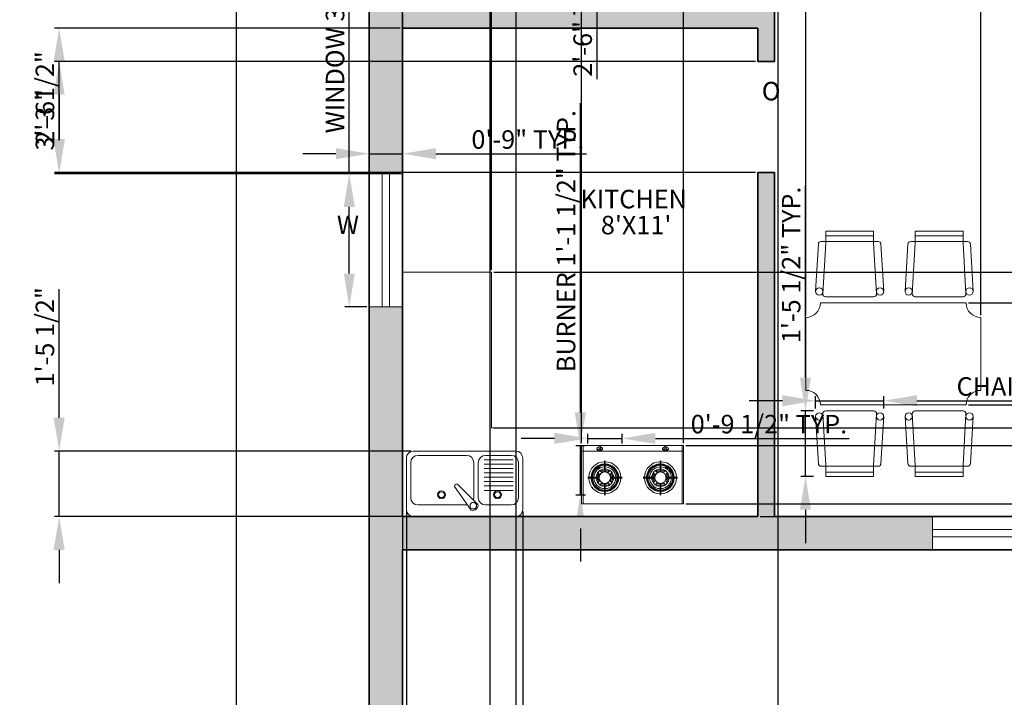
# Model space of a CAD drawing. Units: inches. Extents: x 2265 to 2807, y 1544 to 2401.
# Tile 2 of 9: x 2265 to 2531, y 1890 to 2073. Entities that reach past the tile are written whole.
import ezdxf

# ---------------------------------------------------------------- set-up
doc = ezdxf.new("R2010")
doc.units = ezdxf.units.IN
for name, color, linetype, lineweight in [('A-ANNO-DIMS', 2, 'Continuous', 18), ('A-ANNO-TEXT', 7, 'Continuous', 18), ('A-AREA-IDEN', 7, 'Continuous', 18), ('A-EQPM', 8, 'Continuous', 15), ('A-FLOR-CASE', 8, 'Continuous', 20), ('A-FLOR-FIXT', 8, 'Continuous', 18), ('A-GLAZ', 4, 'Continuous', 18), ('A-WALL', 7, 'Continuous', 35), ('A-WALL-PATT', 18, 'Continuous', 13), ('C-PROP', 7, 'Continuous', 25), ('Furniture', 161, 'Continuous', 15)]:
    doc.layers.add(name, color=color, linetype=linetype, lineweight=lineweight)
doc.styles.add('ARIAL', font='times.ttf', dxfattribs={"height": 5})
doc.styles.get("Standard").update_dxf_attribs({"font": 'arial.ttf', "height": 5})
doc.dimstyles.new('ISO-25', dxfattribs={"dimtxt": 5, "dimasz": 9, "dimexe": 1.25, "dimexo": 0.625, "dimtad": 1, "dimlunit": 3, "dimtxsty": 'Standard', "dimcen": 2.5, "dimadec": 0, "dimazin": 0, "dimtfac": 1, "dimtmove": 0, "dimatfit": 3, "dimfxl": 1, "dimarcsym": 0})

# ---------------------------------------------------------------- blocks, each defined once
blk = doc.blocks.new('GLAZING-48IN')
for p, q in [((48, 9), (0, 9)), ((0, 5.5), (48, 5.5)), ((0, 5.5), (48, 5.5)), ((0, 3.5), (48, 3.5)), ((0, 0), (48, 0))]:
    blk.add_line(p, q)
blk = doc.blocks.new('GLAZING-36IN')
for p, q in [((0, 36), (0, 0)), ((3.5, 36), (3.5, 0)), ((5.5, 36), (5.5, 0)), ((5.5, 36), (5.5, 0)), ((9, 0), (9, 36))]:
    blk.add_line(p, q)
blk = doc.blocks.new('DINING-CHAIR')
for p, q in [((0, 16.18), (0.74, 3.5)), ((1.93, 16.88), (2.73, 3.09)), ((2.72, 17.72), (15.66, 17.72)), ((16.45, 16.88), (15.65, 3.09)), ((18.38, 16.18), (17.65, 3.5)), ((1.52, 2.76), (16.86, 2.76)), ((2.72, 0), (2.73, 3.09)), ((15.66, 0), (15.65, 3.09)), ((2.72, 1.18), (15.66, 1.18)), ((2.72, 0), (15.66, 0))]:
    blk.add_line(p, q)
for centre in [(0.98, 16.24), (17.39, 16.24)]:
    blk.add_circle(centre, 0.984)
for centre, start, end in [((2.72, 16.93), 90, 183.3132), ((15.66, 16.93), 356.6868, 90), ((1.52, 3.54), 183.3132, 270), ((1.52, 3.54), 183.3132, 270), ((16.86, 3.54), 270, 356.6868)]:
    blk.add_arc(centre, 0.787, start, end)
blk = doc.blocks.new('HOB-BURNER-CONTROL')
for p, q in [((2.48, 12.56), (2.48, 12.42)), ((3.09, 13.22), (3.09, 12.56)), ((3.09, 12.56), (3.09, 12.34)), ((3.36, 13.3), (3.17, 13.3)), ((3.17, 12.48), (3.36, 12.48)), ((3.44, 12.56), (3.44, 13.22)), ((3.44, 12.56), (3.44, 12.34)), ((4.03, 12.56), (4.03, 12.42)), ((4.54, 6.45), (4.54, 9.28)), ((4.73, 6.45), (4.73, 9.28)), ((2.54, 5.77), (2.75, 5.57)), ((2.71, 6.05), (3.13, 5.62)), ((3.27, 6.61), (3.69, 6.18)), ((3.54, 6.78), (3.75, 6.57)), ((5.73, 6.78), (5.52, 6.57)), ((6, 6.61), (5.58, 6.18)), ((6.56, 6.05), (6.13, 5.62)), ((6.73, 5.77), (6.52, 5.57)), ((2.87, 4.78), (0, 4.78)), ((2.87, 4.58), (0, 4.58)), ((2.75, 3.79), (2.54, 3.59)), ((3.13, 3.74), (2.71, 3.31)), ((3.69, 3.18), (3.27, 2.76)), ((3.75, 2.79), (3.54, 2.59)), ((4.54, 2.91), (4.54, 0)), ((4.73, 2.91), (4.73, 0)), ((5.52, 2.79), (5.73, 2.59)), ((5.58, 3.18), (6, 2.76)), ((6.13, 3.74), (6.56, 3.31)), ((6.4, 4.78), (9.3, 4.78)), ((6.4, 4.58), (9.3, 4.58)), ((6.52, 3.79), (6.73, 3.59))]:
    blk.add_line(p, q)
for centre, radius in [((2.72, 7.23), 0.141), ((3.08, 7.46), 0.141), ((4.63, 4.68), 1.54)]:
    blk.add_circle(centre, radius)
for centre, radius, start, end in [((2.55, 12.57), 0.0787, 165.3271, 228.6514), ((3.25, 13.37), 1.14, 228.6514, 256.6925), ((3.01, 12.34), 0.0787, 256.6925, 0), ((3.17, 13.22), 0.0787, 90, 180), ((3.17, 12.56), 0.0787, 180, 270), ((3.36, 13.22), 0.0787, 0, 90), ((3.36, 12.56), 0.0787, 270, 0), ((3.52, 12.34), 0.0787, 180, 284.376), ((3.25, 13.37), 1.14, 284.376, 309.6111), ((3.93, 12.58), 0.104, 300.0749, 32.1858), ((4.63, 4.68), 4.33, 91.3023, 178.6977), ((4.63, 4.68), 3.74, 91.5918, 178.4082), ((4.63, 4.68), 3.54, 91.5918, 178.4082), ((4.63, 4.68), 3.35, 91.6854, 178.3146), ((4.63, 4.68), 4.33, 1.3023, 88.6977), ((4.63, 4.68), 3.54, 1.5918, 88.4082), ((4.63, 4.68), 3.35, 1.6854, 88.3146), ((4.63, 4.68), 3.74, 1.5918, 88.4082), ((4.63, 4.68), 2.95, 91.9102, 178.0898), ((4.63, 4.68), 2.36, 92.388, 177.612), ((4.63, 4.68), 2.09, 154.8539, 177.2964), ((4.63, 4.68), 1.77, 147.8396, 176.8153), ((4.63, 4.68), 1.77, 93.1847, 122.1604), ((4.63, 4.68), 2.09, 92.7036, 115.1461), ((4.63, 6.48), 0.104, 198.751, 341.249), ((4.63, 4.68), 2.95, 1.9102, 88.0898), ((4.63, 4.68), 2.36, 2.388, 87.612), ((4.63, 4.68), 2.09, 64.8539, 87.2964), ((4.63, 4.68), 1.77, 57.8396, 86.8153), ((4.63, 4.68), 1.77, 3.1847, 32.1604), ((4.63, 4.68), 2.09, 2.7036, 25.1461), ((4.63, 4.68), 4.33, 181.3023, 268.6977), ((4.63, 4.68), 3.74, 181.5918, 268.4082), ((4.63, 4.68), 3.54, 181.5918, 268.4082), ((4.63, 4.68), 3.35, 181.6854, 268.3146), ((4.63, 4.68), 2.95, 181.9102, 268.0898), ((4.63, 4.68), 2.36, 182.388, 267.612), ((4.63, 4.68), 2.09, 182.7036, 205.1461), ((2.85, 4.68), 0.0991, 276.7354, 83.2646), ((4.63, 4.68), 1.77, 183.1847, 212.1604), ((4.63, 4.68), 1.77, 237.8396, 266.8153), ((4.63, 4.68), 2.09, 244.8539, 267.2964), ((4.63, 2.88), 0.105, 20.5507, 159.4493), ((4.63, 4.68), 4.33, 271.3023, 358.6977), ((4.63, 4.68), 3.54, 271.5918, 358.4082), ((4.63, 4.68), 3.35, 271.6854, 358.3146), ((4.63, 4.68), 2.36, 272.388, 357.612), ((4.63, 4.68), 2.95, 271.9102, 358.0898), ((4.63, 4.68), 1.77, 273.1847, 302.1604), ((4.63, 4.68), 2.09, 272.7036, 295.1461), ((4.63, 4.68), 3.74, 271.5918, 358.4082), ((4.63, 4.68), 1.77, 327.8396, 356.8153), ((6.44, 4.68), 0.106, 111.7885, 248.2115), ((4.63, 4.68), 2.09, 334.8539, 357.2964)]:
    blk.add_arc(centre, radius, start, end)
at = {"extrusion": (0, 0, -1)}
for start_param, end_param in [(0.167831, 1.359229), (3.311147, 6.113631), (1.807364, 2.885846)]:
    blk.add_ellipse((3.25, 12.51), major_axis=(-0.788, 0), ratio=0.647058, start_param=start_param, end_param=end_param, dxfattribs=at)
blk = doc.blocks.new('*D17')
at = {"layer": 'A-ANNO-DIMS', "color": 0, "lineweight": -2, "transparency": 16777216}
for p, q in [((2353.7, 2031.88), (2353.7, 2105.4)), ((2358.48, 2031.88), (2352.45, 2031.88)), ((2353.7, 2004.88), (2353.7, 2022.88)), ((2358.48, 1995.88), (2352.45, 1995.88))]:
    blk.add_line(p, q, dxfattribs=at)
at = {"layer": 'A-ANNO-DIMS', "color": 0, "lineweight": 100, "transparency": 16777216}
for points in [[(2352.2, 2022.88), (2355.2, 2022.88), (2353.7, 2031.88)], [(2352.2, 2004.88), (2355.2, 2004.88), (2353.7, 1995.88)]]:
    blk.add_solid(points, dxfattribs=at)
at = {"layer": 'Defpoints', "color": 0, "lineweight": 100, "transparency": 16777216}
for p in [(2353.7, 2031.88), (2359.1, 2031.88), (2359.1, 1995.88)]:
    blk.add_point(p, dxfattribs=at)
at = {"layer": 'A-ANNO-DIMS', "color": 0, "transparency": 16777216, "insert": (2350.49, 2073.14), "char_height": 5, "attachment_point": 5, "rotation": 90}
blk.add_mtext('WINDOW 3\'-0" TYP.', dxfattribs=at)
blk = doc.blocks.new('*D18')
at = {"layer": 'A-ANNO-DIMS', "color": 0, "lineweight": -2, "transparency": 16777216}
for p, q in [((2359.1, 2032.51), (2359.1, 2038.53)), ((2368.1, 2032.51), (2368.1, 2038.53)), ((2350.1, 2037.28), (2341.1, 2037.28)), ((2359.1, 2037.28), (2368.1, 2037.28)), ((2377.1, 2037.28), (2417.83, 2037.28))]:
    blk.add_line(p, q, dxfattribs=at)
at = {"layer": 'A-ANNO-DIMS', "color": 0, "lineweight": 100, "transparency": 16777216}
for points in [[(2350.1, 2038.78), (2350.1, 2035.78), (2359.1, 2037.28)], [(2377.1, 2038.78), (2377.1, 2035.78), (2368.1, 2037.28)]]:
    blk.add_solid(points, dxfattribs=at)
at = {"layer": 'Defpoints', "color": 0, "lineweight": 100, "transparency": 16777216}
for p in [(2368.1, 2037.28), (2359.1, 2031.88), (2368.1, 2031.88)]:
    blk.add_point(p, dxfattribs=at)
at = {"layer": 'A-ANNO-DIMS', "color": 0, "transparency": 16777216, "insert": (2401.96, 2040.46), "char_height": 5, "attachment_point": 5}
blk.add_mtext('0\'-9" TYP.', dxfattribs=at)
blk = doc.blocks.new('*D24')
at = {"layer": 'A-ANNO-DIMS', "color": 0, "lineweight": -2, "transparency": 16777216}
for p, q in [((2424.48, 2128.23), (2419.35, 2128.23)), ((2420.6, 2119.23), (2420.6, 2107.23)), ((2424.48, 2098.23), (2419.35, 2098.23)), ((2420.6, 2098.23), (2420.6, 2057.42))]:
    blk.add_line(p, q, dxfattribs=at)
at = {"layer": 'A-ANNO-DIMS', "color": 0, "lineweight": 100, "transparency": 16777216}
for points in [[(2419.1, 2119.23), (2422.1, 2119.23), (2420.6, 2128.23)], [(2419.1, 2107.23), (2422.1, 2107.23), (2420.6, 2098.23)]]:
    blk.add_solid(points, dxfattribs=at)
at = {"layer": 'Defpoints', "color": 0, "lineweight": 100, "transparency": 16777216}
for p in [(2425.1, 2128.23), (2420.6, 2098.23), (2425.1, 2098.23)]:
    blk.add_point(p, dxfattribs=at)
at = {"layer": 'A-ANNO-DIMS', "color": 0, "transparency": 16777216, "insert": (2417.42, 2073.33), "char_height": 5, "attachment_point": 5, "rotation": 90}
blk.add_mtext('2\'-6" TYP.', dxfattribs=at)
blk = doc.blocks.new('*D27')
at = {"layer": 'A-ANNO-DIMS', "color": 0, "lineweight": -2, "transparency": 16777216}
for p, q in [((2470.74, 1970.54), (2461.74, 1970.54)), ((2479.74, 1968.41), (2479.74, 1971.79)), ((2479.74, 1970.54), (2498.12, 1970.54)), ((2498.12, 1968.41), (2498.12, 1971.79)), ((2507.12, 1970.54), (2583.11, 1970.54))]:
    blk.add_line(p, q, dxfattribs=at)
at = {"layer": 'A-ANNO-DIMS', "color": 0, "lineweight": 100, "transparency": 16777216}
for points in [[(2470.74, 1972.04), (2470.74, 1969.04), (2479.74, 1970.54)], [(2507.12, 1972.04), (2507.12, 1969.04), (2498.12, 1970.54)]]:
    blk.add_solid(points, dxfattribs=at)
at = {"layer": 'Defpoints', "color": 0, "lineweight": 100, "transparency": 16777216}
for p in [(2498.12, 1970.54), (2479.74, 1967.79), (2498.12, 1967.79)]:
    blk.add_point(p, dxfattribs=at)
at = {"layer": 'A-ANNO-DIMS', "color": 0, "transparency": 16777216, "insert": (2549.62, 1973.75), "char_height": 5, "attachment_point": 5}
blk.add_mtext('CHAIR 1\'-6 1/2" TYP.', dxfattribs=at)
blk = doc.blocks.new('*D28')
at = {"layer": 'A-ANNO-DIMS', "color": 0, "lineweight": -2, "transparency": 16777216}
for p, q in [((2476.98, 1976.79), (2476.98, 2028.69)), ((2479.11, 1967.79), (2475.73, 1967.79)), ((2476.98, 1950.07), (2476.98, 1967.79)), ((2479.11, 1950.07), (2475.73, 1950.07)), ((2476.98, 1941.07), (2476.98, 1932.07))]:
    blk.add_line(p, q, dxfattribs=at)
at = {"layer": 'A-ANNO-DIMS', "color": 0, "lineweight": 100, "transparency": 16777216}
for points in [[(2475.48, 1976.79), (2478.48, 1976.79), (2476.98, 1967.79)], [(2475.48, 1941.07), (2478.48, 1941.07), (2476.98, 1950.07)]]:
    blk.add_solid(points, dxfattribs=at)
at = {"layer": 'Defpoints', "color": 0, "lineweight": 100, "transparency": 16777216}
for p in [(2476.98, 1967.79), (2479.74, 1967.79), (2479.74, 1950.07)]:
    blk.add_point(p, dxfattribs=at)
at = {"layer": 'A-ANNO-DIMS', "color": 0, "transparency": 16777216, "insert": (2473.77, 2007.24), "char_height": 5, "attachment_point": 5, "rotation": 90}
blk.add_mtext('1\'-5 1/2" TYP.', dxfattribs=at)
blk = doc.blocks.new('*D33')
at = {"layer": 'A-ANNO-DIMS', "color": 0, "lineweight": -2, "transparency": 16777216}
for p, q in [((2416.14, 1967.36), (2416.14, 2050.96)), ((2417.51, 1958.36), (2414.89, 1958.36)), ((2416.14, 1945.06), (2416.14, 1958.36)), ((2417.51, 1945.06), (2414.89, 1945.06)), ((2416.14, 1936.06), (2416.14, 1927.06))]:
    blk.add_line(p, q, dxfattribs=at)
at = {"layer": 'A-ANNO-DIMS', "color": 0, "lineweight": 100, "transparency": 16777216}
for points in [[(2414.64, 1967.36), (2417.64, 1967.36), (2416.14, 1958.36)], [(2414.64, 1936.06), (2417.64, 1936.06), (2416.14, 1945.06)]]:
    blk.add_solid(points, dxfattribs=at)
at = {"layer": 'Defpoints', "color": 0, "lineweight": 100, "transparency": 16777216}
for p in [(2416.14, 1958.36), (2418.13, 1958.36), (2418.13, 1945.06)]:
    blk.add_point(p, dxfattribs=at)
at = {"layer": 'A-ANNO-DIMS', "color": 0, "transparency": 16777216, "insert": (2412.93, 2013.66), "char_height": 5, "attachment_point": 5, "rotation": 90}
blk.add_mtext('BURNER 1\'-1 1/2" TYP.', dxfattribs=at)
blk = doc.blocks.new('*D34')
at = {"layer": 'A-ANNO-DIMS', "color": 0, "lineweight": -2, "transparency": 16777216}
for p, q in [((2418.13, 1958.99), (2418.13, 1961.61)), ((2427.43, 1958.99), (2427.43, 1961.61)), ((2409.13, 1960.36), (2400.13, 1960.36)), ((2418.13, 1960.36), (2427.43, 1960.36)), ((2436.43, 1960.36), (2488.81, 1960.36))]:
    blk.add_line(p, q, dxfattribs=at)
at = {"layer": 'A-ANNO-DIMS', "color": 0, "lineweight": 100, "transparency": 16777216}
for points in [[(2409.13, 1961.86), (2409.13, 1958.86), (2418.13, 1960.36)], [(2436.43, 1961.86), (2436.43, 1958.86), (2427.43, 1960.36)]]:
    blk.add_solid(points, dxfattribs=at)
at = {"layer": 'Defpoints', "color": 0, "lineweight": 100, "transparency": 16777216}
for p in [(2427.43, 1960.36), (2418.13, 1958.36), (2427.43, 1958.36)]:
    blk.add_point(p, dxfattribs=at)
at = {"layer": 'A-ANNO-DIMS', "color": 0, "transparency": 16777216, "insert": (2467.12, 1963.57), "char_height": 5, "attachment_point": 5}
blk.add_mtext('0\'-9 1/2" TYP.', dxfattribs=at)
blk = doc.blocks.new('*D37')
at = {"layer": 'A-ANNO-DIMS', "color": 0, "lineweight": -2, "transparency": 16777216}
for p, q in [((2463.48, 2062.23), (2274.04, 2062.23)), ((2275.29, 2053.23), (2275.29, 2041.23)), ((2463.48, 2032.23), (2274.04, 2032.23))]:
    blk.add_line(p, q, dxfattribs=at)
at = {"layer": 'A-ANNO-DIMS', "color": 0, "lineweight": 100, "transparency": 16777216}
for points in [[(2273.79, 2053.23), (2276.79, 2053.23), (2275.29, 2062.23)], [(2273.79, 2041.23), (2276.79, 2041.23), (2275.29, 2032.23)]]:
    blk.add_solid(points, dxfattribs=at)
at = {"layer": 'Defpoints', "color": 0, "lineweight": 100, "transparency": 16777216}
for p in [(2464.1, 2062.23), (2275.29, 2032.23), (2464.1, 2032.23)]:
    blk.add_point(p, dxfattribs=at)
at = {"layer": 'A-ANNO-DIMS', "color": 0, "transparency": 16777216, "insert": (2272.11, 2047.23), "char_height": 5, "attachment_point": 5, "rotation": 90}
blk.add_mtext('2\'-6"', dxfattribs=at)
blk = doc.blocks.new('*D40')
at = {"layer": 'A-ANNO-DIMS', "color": 0, "lineweight": -2, "transparency": 16777216}
for p, q in [((2368.1, 2005.86), (2368.1, 2297.59)), ((2392.1, 2005.86), (2392.1, 2297.59)), ((2377.1, 2296.34), (2383.1, 2296.34))]:
    blk.add_line(p, q, dxfattribs=at)
at = {"layer": 'A-ANNO-DIMS', "color": 0, "lineweight": 100, "transparency": 16777216}
for points in [[(2377.1, 2297.84), (2377.1, 2294.84), (2368.1, 2296.34)], [(2383.1, 2297.84), (2383.1, 2294.84), (2392.1, 2296.34)]]:
    blk.add_solid(points, dxfattribs=at)
at = {"layer": 'Defpoints', "color": 0, "lineweight": 100, "transparency": 16777216}
for p in [(2392.1, 2296.34), (2368.1, 2005.23), (2392.1, 2005.23)]:
    blk.add_point(p, dxfattribs=at)
at = {"layer": 'A-ANNO-DIMS', "color": 0, "transparency": 16777216, "insert": (2380.1, 2299.52), "char_height": 5, "attachment_point": 5}
blk.add_mtext('2\'-0"', dxfattribs=at)
blk = doc.blocks.new('*D41')
at = {"layer": 'A-ANNO-DIMS', "color": 0, "lineweight": -2, "transparency": 16777216}
for p, q in [((2392.73, 2005.23), (2804.46, 2005.23)), ((2803.21, 1996.23), (2803.21, 1972.23)), ((2392.73, 1963.23), (2804.46, 1963.23))]:
    blk.add_line(p, q, dxfattribs=at)
at = {"layer": 'A-ANNO-DIMS', "color": 0, "lineweight": 100, "transparency": 16777216}
for points in [[(2801.71, 1996.23), (2804.71, 1996.23), (2803.21, 2005.23)], [(2801.71, 1972.23), (2804.71, 1972.23), (2803.21, 1963.23)]]:
    blk.add_solid(points, dxfattribs=at)
at = {"layer": 'Defpoints', "color": 0, "lineweight": 100, "transparency": 16777216}
for p in [(2392.1, 2005.23), (2392.1, 1963.23), (2803.21, 1963.23)]:
    blk.add_point(p, dxfattribs=at)
at = {"layer": 'A-ANNO-DIMS', "color": 0, "transparency": 16777216, "insert": (2800.03, 1984.23), "char_height": 5, "attachment_point": 5, "rotation": 90}
blk.add_mtext('3\'-6"', dxfattribs=at)
blk = doc.blocks.new('*D42')
at = {"layer": 'A-ANNO-DIMS', "color": 0, "lineweight": -2, "transparency": 16777216}
for p, q in [((2464.73, 1963.23), (2804.46, 1963.23)), ((2803.21, 1954.23), (2803.21, 1948.23)), ((2464.73, 1939.23), (2804.46, 1939.23))]:
    blk.add_line(p, q, dxfattribs=at)
at = {"layer": 'A-ANNO-DIMS', "color": 0, "lineweight": 100, "transparency": 16777216}
for points in [[(2801.71, 1954.23), (2804.71, 1954.23), (2803.21, 1963.23)], [(2801.71, 1948.23), (2804.71, 1948.23), (2803.21, 1939.23)]]:
    blk.add_solid(points, dxfattribs=at)
at = {"layer": 'Defpoints', "color": 0, "lineweight": 100, "transparency": 16777216}
for p in [(2464.1, 1963.23), (2464.1, 1939.23), (2803.21, 1939.23)]:
    blk.add_point(p, dxfattribs=at)
at = {"layer": 'A-ANNO-DIMS', "color": 0, "transparency": 16777216, "insert": (2800.03, 1951.23), "char_height": 5, "attachment_point": 5, "rotation": 90}
blk.add_mtext('2\'-0"', dxfattribs=at)
blk = doc.blocks.new('*D43')
at = {"layer": 'A-ANNO-DIMS', "color": 0, "lineweight": -2, "transparency": 16777216}
for p, q in [((2416.49, 1959.08), (2416.49, 2297.59)), ((2444.05, 1959.08), (2444.05, 2297.59)), ((2425.49, 2296.34), (2435.05, 2296.34))]:
    blk.add_line(p, q, dxfattribs=at)
at = {"layer": 'A-ANNO-DIMS', "color": 0, "lineweight": 100, "transparency": 16777216}
for points in [[(2425.49, 2297.84), (2425.49, 2294.84), (2416.49, 2296.34)], [(2435.05, 2297.84), (2435.05, 2294.84), (2444.05, 2296.34)]]:
    blk.add_solid(points, dxfattribs=at)
at = {"layer": 'Defpoints', "color": 0, "lineweight": 100, "transparency": 16777216}
for p in [(2444.05, 2296.34), (2416.49, 1958.45), (2444.05, 1958.45)]:
    blk.add_point(p, dxfattribs=at)
at = {"layer": 'A-ANNO-DIMS', "color": 0, "transparency": 16777216, "insert": (2430.27, 2299.56), "char_height": 5, "attachment_point": 5}
blk.add_mtext('2\'-3 1/2"', dxfattribs=at)
blk = doc.blocks.new('*D44')
at = {"layer": 'A-ANNO-DIMS', "color": 0, "lineweight": -2, "transparency": 16777216}
for p, q in [((2369.12, 1940.58), (2369.12, 1546.93)), ((2400.62, 1940.58), (2400.62, 1546.93)), ((2378.12, 1548.18), (2391.62, 1548.18))]:
    blk.add_line(p, q, dxfattribs=at)
at = {"layer": 'A-ANNO-DIMS', "color": 0, "lineweight": 100, "transparency": 16777216}
for points in [[(2378.12, 1549.68), (2378.12, 1546.68), (2369.12, 1548.18)], [(2391.62, 1549.68), (2391.62, 1546.68), (2400.62, 1548.18)]]:
    blk.add_solid(points, dxfattribs=at)
at = {"layer": 'Defpoints', "color": 0, "lineweight": 100, "transparency": 16777216}
for p in [(2369.12, 1941.2), (2400.62, 1941.2), (2400.62, 1548.18)]:
    blk.add_point(p, dxfattribs=at)
at = {"layer": 'A-ANNO-DIMS', "color": 0, "transparency": 16777216, "insert": (2384.87, 1551.4), "char_height": 5, "attachment_point": 5}
blk.add_mtext('2\'-7 1/2"', dxfattribs=at)
blk = doc.blocks.new('*D45')
at = {"layer": 'A-ANNO-DIMS', "color": 0, "lineweight": -2, "transparency": 16777216}
for p, q in [((2391.72, 2088.38), (2391.72, 1546.93)), ((2368.1, 2075.11), (2368.1, 1546.93)), ((2377.1, 1548.18), (2382.72, 1548.18)), ((2391.72, 1548.18), (2430.33, 1548.18))]:
    blk.add_line(p, q, dxfattribs=at)
at = {"layer": 'A-ANNO-DIMS', "color": 0, "lineweight": 100, "transparency": 16777216}
for points in [[(2377.1, 1549.68), (2377.1, 1546.68), (2368.1, 1548.18)], [(2382.72, 1549.68), (2382.72, 1546.68), (2391.72, 1548.18)]]:
    blk.add_solid(points, dxfattribs=at)
at = {"layer": 'Defpoints', "color": 0, "lineweight": 100, "transparency": 16777216}
for p in [(2391.72, 2089), (2368.1, 2075.73), (2391.72, 1548.18)]:
    blk.add_point(p, dxfattribs=at)
at = {"layer": 'A-ANNO-DIMS', "color": 0, "transparency": 16777216, "insert": (2415.53, 1551.4), "char_height": 5, "attachment_point": 5}
blk.add_mtext('1\'-11 1/2"', dxfattribs=at)
blk = doc.blocks.new('*D46')
at = {"layer": 'A-ANNO-DIMS', "color": 0, "lineweight": -2, "transparency": 16777216}
for p, q in [((2803.21, 2104.95), (2803.21, 2128.02)), ((2381.23, 2095.95), (2804.46, 2095.95)), ((2803.21, 2082.06), (2803.21, 2095.95)), ((2381.23, 2082.06), (2804.46, 2082.06)), ((2803.21, 2073.06), (2803.21, 2064.06))]:
    blk.add_line(p, q, dxfattribs=at)
at = {"layer": 'A-ANNO-DIMS', "color": 0, "lineweight": 100, "transparency": 16777216}
for points in [[(2801.71, 2104.95), (2804.71, 2104.95), (2803.21, 2095.95)], [(2801.71, 2073.06), (2804.71, 2073.06), (2803.21, 2082.06)]]:
    blk.add_solid(points, dxfattribs=at)
at = {"layer": 'Defpoints', "color": 0, "lineweight": 100, "transparency": 16777216}
for p in [(2380.61, 2095.95), (2803.21, 2095.95), (2380.61, 2082.06)]:
    blk.add_point(p, dxfattribs=at)
at = {"layer": 'A-ANNO-DIMS', "color": 0, "transparency": 16777216, "insert": (2800.07, 2120.99), "char_height": 5, "attachment_point": 5, "rotation": 90}
blk.add_mtext('1\'-2"', dxfattribs=at)
blk = doc.blocks.new('*D48')
at = {"layer": 'A-ANNO-DIMS', "color": 0, "lineweight": -2, "transparency": 16777216}
for p, q in [((2367.48, 2071.23), (2274.04, 2071.23)), ((2275.29, 2040.88), (2275.29, 2062.23)), ((2367.48, 2031.88), (2274.04, 2031.88))]:
    blk.add_line(p, q, dxfattribs=at)
at = {"layer": 'A-ANNO-DIMS', "color": 0, "lineweight": 100, "transparency": 16777216}
for points in [[(2273.79, 2062.23), (2276.79, 2062.23), (2275.29, 2071.23)], [(2273.79, 2040.88), (2276.79, 2040.88), (2275.29, 2031.88)]]:
    blk.add_solid(points, dxfattribs=at)
at = {"layer": 'Defpoints', "color": 0, "lineweight": 100, "transparency": 16777216}
for p in [(2275.29, 2071.23), (2368.1, 2071.23), (2368.1, 2031.88)]:
    blk.add_point(p, dxfattribs=at)
at = {"layer": 'A-ANNO-DIMS', "color": 0, "transparency": 16777216, "insert": (2272.08, 2051.56), "char_height": 5, "attachment_point": 5, "rotation": 90}
blk.add_mtext('3\'-3 1/2"', dxfattribs=at)
blk = doc.blocks.new('*D50')
at = {"layer": 'A-ANNO-DIMS', "color": 0, "lineweight": -2, "transparency": 16777216}
for p, q in [((2398.67, 2169.19), (2398.67, 1546.93)), ((2469.53, 2169.19), (2469.53, 1546.93)), ((2407.67, 1548.18), (2460.53, 1548.18))]:
    blk.add_line(p, q, dxfattribs=at)
at = {"layer": 'A-ANNO-DIMS', "color": 0, "lineweight": 100, "transparency": 16777216}
for points in [[(2407.67, 1549.68), (2407.67, 1546.68), (2398.67, 1548.18)], [(2460.53, 1549.68), (2460.53, 1546.68), (2469.53, 1548.18)]]:
    blk.add_solid(points, dxfattribs=at)
at = {"layer": 'Defpoints', "color": 0, "lineweight": 100, "transparency": 16777216}
for p in [(2398.67, 2169.81), (2469.53, 2169.81), (2469.53, 1548.18)]:
    blk.add_point(p, dxfattribs=at)
at = {"layer": 'A-ANNO-DIMS', "color": 0, "transparency": 16777216, "insert": (2434.1, 1551.36), "char_height": 5, "attachment_point": 5}
blk.add_mtext('5\'-11"', dxfattribs=at)
blk = doc.blocks.new('*D61')
at = {"layer": 'A-ANNO-DIMS', "color": 0, "lineweight": -2, "transparency": 16777216}
for p, q in [((2803.21, 1967.45), (2803.21, 1976.45)), ((2444.67, 1958.45), (2804.46, 1958.45)), ((2803.21, 1958.45), (2803.21, 1942.7)), ((2444.67, 1942.7), (2804.46, 1942.7)), ((2803.21, 1933.7), (2803.21, 1898.98))]:
    blk.add_line(p, q, dxfattribs=at)
at = {"layer": 'A-ANNO-DIMS', "color": 0, "lineweight": 100, "transparency": 16777216}
for points in [[(2801.71, 1967.45), (2804.71, 1967.45), (2803.21, 1958.45)], [(2801.71, 1933.7), (2804.71, 1933.7), (2803.21, 1942.7)]]:
    blk.add_solid(points, dxfattribs=at)
at = {"layer": 'Defpoints', "color": 0, "lineweight": 100, "transparency": 16777216}
for p in [(2444.05, 1958.45), (2444.05, 1942.7), (2803.21, 1942.7)]:
    blk.add_point(p, dxfattribs=at)
at = {"layer": 'A-ANNO-DIMS', "color": 0, "transparency": 16777216, "insert": (2800, 1911.84), "char_height": 5, "attachment_point": 5, "rotation": 90}
blk.add_mtext('1\'-3 1/2"', dxfattribs=at)
blk = doc.blocks.new('*D62')
at = {"layer": 'A-ANNO-DIMS', "color": 0, "lineweight": -2, "transparency": 16777216}
for p, q in [((2275.29, 1965.95), (2275.29, 2000.67)), ((2370.46, 1956.95), (2274.04, 1956.95)), ((2275.29, 1939.23), (2275.29, 1956.95)), ((2370.46, 1939.23), (2274.04, 1939.23)), ((2275.29, 1930.23), (2275.29, 1921.23))]:
    blk.add_line(p, q, dxfattribs=at)
at = {"layer": 'A-ANNO-DIMS', "color": 0, "lineweight": 100, "transparency": 16777216}
for points in [[(2273.79, 1965.95), (2276.79, 1965.95), (2275.29, 1956.95)], [(2273.79, 1930.23), (2276.79, 1930.23), (2275.29, 1939.23)]]:
    blk.add_solid(points, dxfattribs=at)
at = {"layer": 'Defpoints', "color": 0, "lineweight": 100, "transparency": 16777216}
for p in [(2275.29, 1956.95), (2371.09, 1956.95), (2371.09, 1939.23)]:
    blk.add_point(p, dxfattribs=at)
at = {"layer": 'A-ANNO-DIMS', "color": 0, "transparency": 16777216, "insert": (2272.08, 1987.81), "char_height": 5, "attachment_point": 5, "rotation": 90}
blk.add_mtext('1\'-5 1/2"', dxfattribs=at)
blk = doc.blocks.new('*D63')
at = {"layer": 'A-ANNO-DIMS', "color": 0, "lineweight": -2, "transparency": 16777216}
for p, q in [((2477.1, 1993.66), (2477.1, 2297.59)), ((2524.34, 1993.66), (2524.34, 2297.59)), ((2486.1, 2296.34), (2515.34, 2296.34))]:
    blk.add_line(p, q, dxfattribs=at)
at = {"layer": 'A-ANNO-DIMS', "color": 0, "lineweight": 100, "transparency": 16777216}
for points in [[(2486.1, 2297.84), (2486.1, 2294.84), (2477.1, 2296.34)], [(2515.34, 2297.84), (2515.34, 2294.84), (2524.34, 2296.34)]]:
    blk.add_solid(points, dxfattribs=at)
at = {"layer": 'Defpoints', "color": 0, "lineweight": 100, "transparency": 16777216}
for p in [(2524.34, 2296.34), (2477.1, 1993.03), (2524.34, 1993.03)]:
    blk.add_point(p, dxfattribs=at)
at = {"layer": 'A-ANNO-DIMS', "color": 0, "transparency": 16777216, "insert": (2500.72, 2299.52), "char_height": 5, "attachment_point": 5}
blk.add_mtext('3\'-11"', dxfattribs=at)
blk = doc.blocks.new('*D64')
at = {"layer": 'A-ANNO-DIMS', "color": 0, "lineweight": -2, "transparency": 16777216}
for p, q in [((2521.03, 1996.97), (2804.46, 1996.97)), ((2803.21, 1978.41), (2803.21, 1987.97)), ((2521.03, 1969.41), (2804.46, 1969.41))]:
    blk.add_line(p, q, dxfattribs=at)
at = {"layer": 'A-ANNO-DIMS', "color": 0, "lineweight": 100, "transparency": 16777216}
for points in [[(2801.71, 1987.97), (2804.71, 1987.97), (2803.21, 1996.97)], [(2801.71, 1978.41), (2804.71, 1978.41), (2803.21, 1969.41)]]:
    blk.add_solid(points, dxfattribs=at)
at = {"layer": 'Defpoints', "color": 0, "lineweight": 100, "transparency": 16777216}
for p in [(2520.4, 1996.97), (2803.21, 1996.97), (2520.4, 1969.41)]:
    blk.add_point(p, dxfattribs=at)
at = {"layer": 'A-ANNO-DIMS', "color": 0, "transparency": 16777216, "insert": (2800, 1983.19), "char_height": 5, "attachment_point": 5, "rotation": 90}
blk.add_mtext('2\'-3 1/2"', dxfattribs=at)

msp = doc.modelspace()

# ---------------------------------------------------------------- hatches: boundary and pattern name
at = {"layer": 'A-WALL-PATT'}
h = msp.add_hatch(color=256, dxfattribs=at)
h.dxf.hatch_style = 1
h.paths.add_polyline_path([(2416.101, 2255.733), (2359.101, 2255.733), (2359.101, 2205.483), (2368.101, 2205.483), (2368.101, 2246.733), (2416.101, 2246.733)])
h.paths.add_polyline_path([(2528.601, 2255.733), (2452.101, 2255.733), (2452.101, 2246.733), (2487.251, 2246.733), (2500.101, 2246.733), (2500.101, 2168.733), (2504.601, 2168.733), (2504.601, 2170.233), (2525.601, 2170.233), (2525.601, 2174.733), (2504.601, 2174.733), (2504.601, 2246.733), (2528.601, 2246.733)])
h.paths.add_polyline_path([(2603.601, 2255.733), (2552.601, 2255.733), (2552.601, 2246.733), (2576.601, 2246.733), (2576.601, 2174.733), (2555.601, 2174.733), (2555.601, 2170.233), (2576.601, 2170.233), (2576.601, 2123.733), (2581.101, 2123.733), (2581.101, 2246.733), (2603.601, 2246.733)])
h.paths.add_polyline_path([(2671.101, 2255.733), (2639.601, 2255.733), (2639.601, 2246.733), (2662.101, 2246.733), (2662.101, 2083.435), (2671.101, 2083.435)])
h.paths.add_polyline_path([(2671.101, 2035.435), (2662.101, 2035.435), (2662.101, 1939.233), (2644.101, 1939.233), (2644.101, 1930.233), (2662.101, 1930.233), (2662.101, 1814.733), (2644.101, 1814.733), (2644.101, 1805.733), (2671.101, 1805.733)])
h.paths.add_polyline_path([(2368.101, 1930.233), (2511.351, 1930.233), (2511.351, 1939.233), (2468.601, 1939.233), (2468.601, 2032.233), (2464.101, 2032.233), (2464.101, 1939.233), (2368.101, 1939.233), (2368.101, 1995.884), (2359.101, 1995.884), (2359.101, 1805.733), (2602.101, 1805.733), (2602.101, 1814.733), (2368.101, 1814.733)])
h.paths.add_polyline_path([(2368.101, 2071.233), (2464.101, 2071.233), (2464.101, 2062.233), (2468.601, 2062.233), (2468.601, 2123.733), (2504.601, 2123.733), (2504.601, 2132.733), (2500.101, 2132.733), (2500.101, 2128.233), (2455.101, 2128.233), (2455.101, 2123.733), (2464.101, 2123.733), (2464.101, 2075.733), (2368.101, 2075.733), (2368.101, 2087.733), (2359.101, 2087.733), (2359.101, 2031.884), (2368.101, 2031.884)])
h.paths.add_polyline_path([(2368.101, 2169.483), (2359.101, 2169.483), (2359.101, 2111.733), (2368.101, 2111.733), (2368.101, 2123.733), (2425.101, 2123.733), (2425.101, 2128.233), (2368.101, 2128.233)])

# ---------------------------------------------------------------- linework, layer by layer
at = {"layer": 'A-EQPM'}
for p, q in [((2416.49, 1958.452), (2416.49, 1942.704)), ((2444.049, 1958.452), (2416.49, 1958.452)), ((2444.049, 1956.877), (2416.49, 1956.877)), ((2416.884, 1958.452), (2416.884, 1942.704)), ((2443.656, 1942.704), (2443.656, 1958.452)), ((2444.049, 1942.704), (2444.049, 1958.452)), ((2416.49, 1942.704), (2444.049, 1942.704))]:
    msp.add_line(p, q, dxfattribs=at)
at = {"layer": 'A-FLOR-CASE'}
for p, q in [((2392.101, 2005.233), (2368.101, 2005.233)), ((2392.101, 1963.233), (2392.101, 2005.233)), ((2464.101, 1963.233), (2392.101, 1963.233))]:
    msp.add_line(p, q, dxfattribs=at)
at = {"layer": 'A-FLOR-FIXT'}
for p, q in [((2398.647, 1956.95), (2371.088, 1956.95)), ((2369.119, 1954.981), (2369.119, 1941.202)), ((2370.3, 1953.8), (2370.3, 1944.351)), ((2385.407, 1955.769), (2372.269, 1955.769)), ((2387.375, 1944.351), (2387.375, 1953.8)), ((2388.556, 1944.351), (2388.556, 1953.8)), ((2390.14, 1954.594), (2398.028, 1954.594)), ((2390.14, 1953.413), (2398.028, 1953.413)), ((2397.466, 1955.769), (2390.525, 1955.769)), ((2399.434, 1944.351), (2399.434, 1953.8)), ((2400.615, 1941.202), (2400.615, 1954.981)), ((2390.14, 1952.232), (2398.028, 1952.232)), ((2390.14, 1951.051), (2398.028, 1951.051)), ((2390.14, 1949.87), (2398.028, 1949.87)), ((2390.14, 1948.689), (2398.028, 1948.689)), ((2386.673, 1940.999), (2382.285, 1947.134)), ((2388.469, 1942.534), (2383.091, 1947.823)), ((2390.14, 1947.507), (2398.028, 1947.507)), ((2390.14, 1946.326), (2398.028, 1946.326)), ((2372.269, 1942.383), (2385.407, 1942.383)), ((2397.466, 1942.383), (2390.525, 1942.383)), ((2371.088, 1939.233), (2398.647, 1939.233))]:
    msp.add_line(p, q, dxfattribs=at)
for centre, radius in [((2378.622, 1945.144), 1.081), ((2378.622, 1945.144), 0.788), ((2393.768, 1945.144), 1.081), ((2393.768, 1945.144), 0.788), ((2387.213, 1942.186), 0.892)]:
    msp.add_circle(centre, radius, dxfattribs=at)
for centre, radius, start, end in [((2371.088, 1954.981), 1.968, 90, 180), ((2398.647, 1954.981), 1.968, 0, 90), ((2372.269, 1953.8), 1.968, 90, 180), ((2385.407, 1953.8), 1.968, 0, 90), ((2390.525, 1953.8), 1.968, 90, 180), ((2397.466, 1953.8), 1.968, 0, 90), ((2382.683, 1947.484), 0.531, 39.73777, 221.31634), ((2372.269, 1944.351), 1.968, 180, 270), ((2385.407, 1944.351), 1.968, 341.10956, 0), ((2390.525, 1944.351), 1.968, 180, 270), ((2397.466, 1944.351), 1.968, 270, 0), ((2371.088, 1941.202), 1.968, 180, 270), ((2385.407, 1944.351), 1.968, 270, 277.6978), ((2387.128, 1942.285), 1.364, 250.52706, 10.52706), ((2398.647, 1941.202), 1.968, 270, 0)]:
    msp.add_arc(centre, radius, start, end, dxfattribs=at)
at = {"layer": 'A-GLAZ'}
for p, q in [((2368.101, 2031.884), (2359.101, 2031.884)), ((2359.101, 1995.884), (2368.101, 1995.884)), ((2511.351, 1939.233), (2511.351, 1930.233))]:
    msp.add_line(p, q, dxfattribs=at)
at = {"layer": 'A-WALL'}
for p, q in [((2359.101, 1805.733), (2359.101, 2255.733)), ((2468.601, 2062.233), (2468.601, 2123.733)), ((2464.101, 2071.233), (2368.101, 2071.233)), ((2368.101, 1939.233), (2368.101, 2071.233)), ((2464.101, 2062.233), (2464.101, 2071.233)), ((2464.101, 2062.233), (2468.601, 2062.233)), ((2464.101, 1939.233), (2464.101, 2032.233)), ((2464.101, 2032.233), (2468.601, 2032.233)), ((2468.601, 1939.233), (2468.601, 2032.233)), ((2464.101, 1939.233), (2368.101, 1939.233)), ((2602.101, 1939.233), (2468.601, 1939.233)), ((2368.101, 1814.733), (2368.101, 1930.233)), ((2602.101, 1930.233), (2368.101, 1930.233))]:
    msp.add_line(p, q, dxfattribs=at)
at = {"layer": 'C-PROP'}
msp.add_line((2323.101, 2255.733), (2323.101, 1805.733), dxfattribs=at)
at = {"layer": 'Furniture'}
for p, q in [((2481.035, 1996.968), (2520.405, 1996.968)), ((2477.098, 1973.346), (2477.098, 1993.031)), ((2524.342, 1993.031), (2524.342, 1973.346)), ((2520.405, 1969.409), (2481.035, 1969.409))]:
    msp.add_line(p, q, dxfattribs=at)
for centre, start, end in [((2477.098, 1996.968), 270, 0), ((2524.342, 1996.968), 180, 270), ((2477.098, 1969.409), 0, 90), ((2524.342, 1969.409), 90, 180)]:
    msp.add_arc(centre, 3.937, start, end, dxfattribs=at)

# ---------------------------------------------------------------- block references
at = {"layer": 'A-EQPM'}
msp.add_blockref('HOB-BURNER-CONTROL', (2418.134, 1945.064), dxfattribs=at)
at = {"layer": 'A-EQPM', "extrusion": (0, 0, -1), "zscale": -1}
msp.add_blockref('HOB-BURNER-CONTROL', (-2442.406, 1945.064), dxfattribs=at)
at = {"layer": 'A-GLAZ'}
for name, p in [('GLAZING-36IN', (2359.101, 1995.884)), ('GLAZING-48IN', (2511.351, 1930.233))]:
    msp.add_blockref(name, p, dxfattribs=at)
at = {"layer": 'Furniture', "extrusion": (0, 0, -1), "zscale": -1, "rotation": 180}
for p in [(-2479.739, 2016.308), (-2503.916, 2016.308)]:
    msp.add_blockref('DINING-CHAIR', p, dxfattribs=at)
at = {"layer": 'Furniture'}
for p in [(2479.739, 1950.069), (2503.916, 1950.069)]:
    msp.add_blockref('DINING-CHAIR', p, dxfattribs=at)

# ---------------------------------------------------------------- texts
at = {"layer": 'A-ANNO-TEXT', "style": 'ARIAL'}
for s, p in [('O', (2465.177, 2051.686)), ('W', (2350.333, 2015.568))]:
    msp.add_text(s, height=5, dxfattribs=at).set_placement(p)
at = {"layer": 'A-AREA-IDEN', "style": 'ARIAL'}
for s, p in [('KITCHEN', (2416.16, 2022.518)), ("8'X11'", (2421.693, 2015.491))]:
    msp.add_text(s, height=5, dxfattribs=at).set_placement(p)

# ---------------------------------------------------------------- dimensions: what is measured, and where the dimension line sits
at = {"layer": 'A-ANNO-DIMS'}
for base, p1, p2, picture, middle in [((2444.049, 2296.343), (2416.49, 1958.452), (2444.049, 1958.452), '*D43', (2430.27, 2299.555)), ((2392.101, 2296.343), (2368.101, 2005.233), (2392.101, 2005.233), '*D40', (2380.101, 2299.521)), ((2524.342, 2296.343), (2477.098, 1993.031), (2524.342, 1993.031), '*D63', (2500.72, 2299.523)), ((2469.534, 1548.185), (2398.668, 2169.812), (2469.534, 2169.812), '*D50', (2434.101, 1551.363)), ((2391.723, 1548.185), (2368.101, 2075.733), (2391.723, 2089.003), '*D45', (2415.526, 1551.395)), ((2400.615, 1548.185), (2369.119, 1941.202), (2400.615, 1941.202), '*D44', (2384.867, 1551.395))]:
    dim = msp.add_linear_dim(base=base, p1=p1, p2=p2, dimstyle='ISO-25', override={"dimdec": 1, "dimlfac": 1, "dimrnd": 0, "dimzin": 1, "dimdsep": 46, "dimlunit": 4, "dimfrac": 2}, dxfattribs=at)
    dim.commit()
    dim.dimension.update_dxf_attribs({"geometry": picture, "text_midpoint": middle})
for base, p1, p2, picture, middle in [((2803.21, 2095.951), (2380.607, 2082.055), (2380.607, 2095.951), '*D46', (2800.075, 2120.986)), ((2275.289, 2071.233), (2368.101, 2031.884), (2368.101, 2071.233), '*D48', (2272.077, 2051.559)), ((2275.289, 2032.233), (2464.101, 2062.233), (2464.101, 2032.233), '*D37', (2272.111, 2047.233)), ((2803.21, 1963.233), (2392.101, 2005.233), (2392.101, 1963.233), '*D41', (2800.03, 1984.233)), ((2275.289, 1956.95), (2371.088, 1939.233), (2371.088, 1956.95), '*D62', (2272.079, 1987.81)), ((2803.21, 1996.968), (2520.405, 1969.409), (2520.405, 1996.968), '*D64', (2799.998, 1983.188)), ((2803.21, 1942.704), (2444.049, 1958.452), (2444.049, 1942.704), '*D61', (2799.998, 1911.843)), ((2803.21, 1939.233), (2464.101, 1963.233), (2464.101, 1939.233), '*D42', (2800.032, 1951.233))]:
    dim = msp.add_linear_dim(base=base, p1=p1, p2=p2, angle=90, dimstyle='ISO-25', override={"dimdec": 1, "dimlfac": 1, "dimrnd": 0, "dimzin": 1, "dimdsep": 46, "dimlunit": 4, "dimfrac": 2}, dxfattribs=at)
    dim.commit()
    dim.dimension.update_dxf_attribs({"geometry": picture, "text_midpoint": middle})
for base, p1, p2, angle, text, picture, middle in [((2420.601, 2098.233), (2425.101, 2128.233), (2425.101, 2098.233), 270, '<> TYP.', '*D24', (2417.423, 2073.327)), ((2353.701, 2031.884), (2359.101, 1995.884), (2359.101, 2031.884), 90, 'WINDOW <> TYP.', '*D17', (2350.488, 2073.144)), ((2416.139, 1958.365), (2418.134, 1945.064), (2418.134, 1958.365), 90, 'BURNER <> TYP.', '*D33', (2412.929, 2013.661)), ((2476.983, 1967.785), (2479.739, 1950.069), (2479.739, 1967.785), 90, '<> TYP.', '*D28', (2473.772, 2007.239))]:
    dim = msp.add_linear_dim(base=base, p1=p1, p2=p2, angle=angle, text=text, dimstyle='ISO-25', override={"dimdec": 1, "dimlfac": 1, "dimrnd": 0, "dimzin": 1, "dimdsep": 46, "dimlunit": 4, "dimfrac": 2}, dxfattribs=at)
    dim.commit()
    dim.dimension.update_dxf_attribs({"geometry": picture, "text_midpoint": middle})
for base, p1, p2, text, picture, middle in [((2368.101, 2037.284), (2359.101, 2031.884), (2368.101, 2031.884), '<> TYP.', '*D18', (2401.965, 2040.462)), ((2498.119, 1970.542), (2479.739, 1967.785), (2498.119, 1967.785), 'CHAIR <> TYP.', '*D27', (2549.616, 1973.753)), ((2427.433, 1960.36), (2418.134, 1958.365), (2427.433, 1958.365), '<> TYP.', '*D34', (2467.123, 1963.57))]:
    dim = msp.add_linear_dim(base=base, p1=p1, p2=p2, text=text, dimstyle='ISO-25', override={"dimdec": 1, "dimlfac": 1, "dimrnd": 0, "dimzin": 1, "dimdsep": 46, "dimlunit": 4, "dimfrac": 2}, dxfattribs=at)
    dim.commit()
    dim.dimension.update_dxf_attribs({"geometry": picture, "text_midpoint": middle})

doc.saveas('drawing.dxf')
